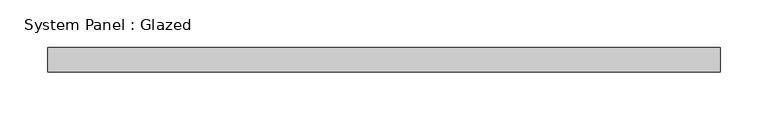
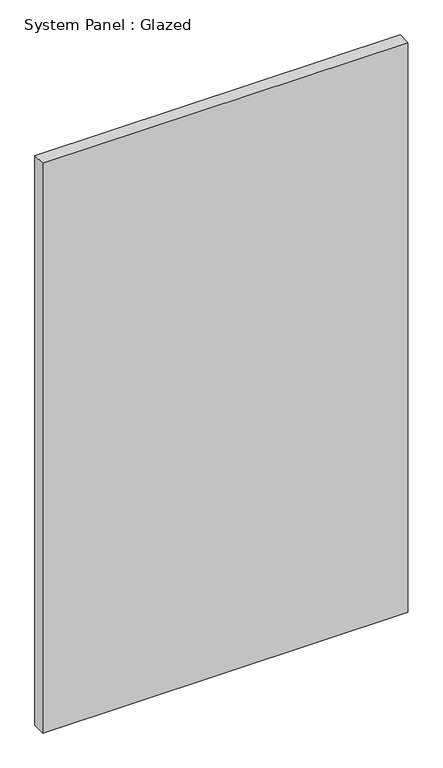
"""IFC4 building model written with IfcOpenShell, lengths in millimetres: plate geometry, System Panel : Glazed."""

from ifc_helpers import new_model, si_unit, origin, origin_with_axes, place, context, project, spatial, polyline, outline, extrude, source, transform, mapped, element, save


def system_panel_glazed_840f75dd(model_context):
    return source(origin(), model_context, "Body", "SweptSolid", [
        extrude(outline(polyline([(350.3083333, 19.05), (-350.3083333, 19.05), (-350.3083333, 44.45), (350.3083333, 44.45), (350.3083333, 19.05)])), origin_with_axes(), (0.0, 0.0, 1.0), 1155.7),
    ])


if __name__ == "__main__":
    model = new_model("IFC4")
    model_context = context("Model", 3, world=origin())
    ifc_project = project(units=[si_unit("LENGTHUNIT", "METRE", prefix="MILLI")], contexts=[model_context])
    site = spatial("IfcSite", under=ifc_project)
    building = spatial("IfcBuilding", under=site)
    placement = place(None, origin())
    system_panel_glazed_shape = system_panel_glazed_840f75dd(model_context)
    element("IfcPlate", 1, ObjectType="System Panel : Glazed", at=placement, inside=building, context=model_context, shape_type="MappedRepresentation", body=[
        mapped(system_panel_glazed_shape, transform((0.0, 0.0, 0.0), x_axis=(1.0, 0.0, 0.0), y_axis=(0.0, 1.0, 0.0), z_axis=(0.0, 0.0, 1.0))),
    ])
    save(model, "model.ifc")

# Revit data of these elements
# Type "System Panel : Glazed"
#   Construction Type Id = "GSP4R"
#   Analytic Construction = "1/8 in Pilkington single glazing"
#   Visual Light Transmittance = 0.9
#   Solar Heat Gain Coefficient = 0.86
#   Heat Transfer Coefficient (U) = 1.18115 BTU/(h·ft²·°F)
# Element 1 (IfcPlate, "System Panel : Glazed")
#   Materials on its faces: "Glass"
# Materials
#   "Glass": class "Glass", colour RGB 0 128 192, transparency 0.75, Description = "Soda Lime Glass", Cost = 0
